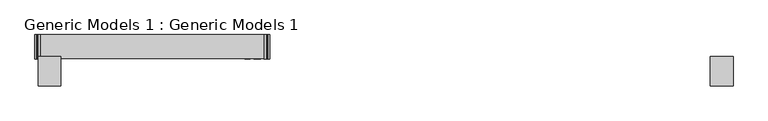
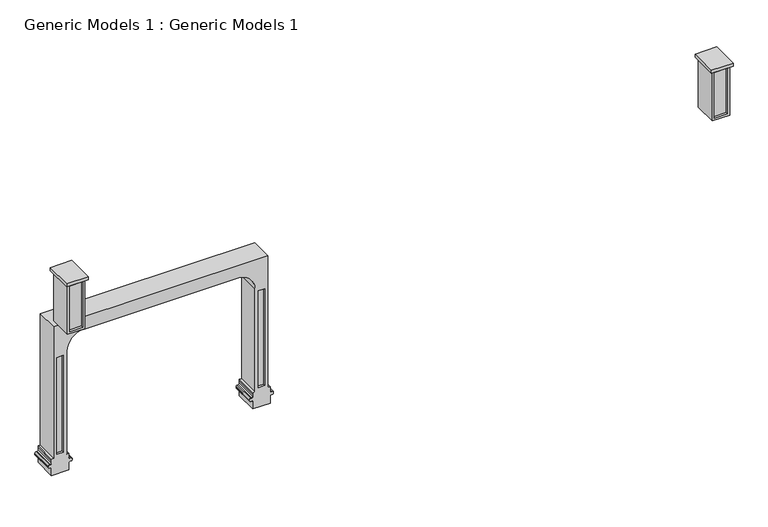
"""IFC4 building model written with IfcOpenShell, lengths in millimetres: proxy geometry, Generic Models 1 : Generic Models 1."""

from ifc_helpers import new_model, si_unit, frame, origin, place, context, project, spatial, polyline, circle_curve, outline, extrude, faceted_brep, source, transform, mapped, element, save
from ifc_brep_helpers import plane_surface, cylinder_surface, revolved_surface, advanced_brep


def generic_models_1_generic_models_1_a6c1d6b2(model_context):
    return source(origin(), model_context, "Body", "SolidModel", [
        advanced_brep(
        [(-3767.7753219, -7793.5697181, 3657.6), (-3767.7753219, -7793.5697181, 406.4), (-3716.9753219, -7793.5697181, 406.4), (-3716.9753219, -7793.5697181, 355.6), (-3716.9753219, -7793.5697181, 304.8), (-3691.5753219, -7793.5697181, 279.4), (-3672.5253219, -7793.5697181, 279.4), (-3640.7753219, -7793.5697181, 247.65), (-3640.7753219, -7793.5697181, 228.6), (-3666.1753219, -7793.5697181, 203.2), (-3695.5632105, -7793.5697181, 203.2), (-3716.9753219, -7793.5697181, 181.7878886), (-3716.9753219, -7793.5697181, 0.0), (-4123.3753219, -7793.5697181, 0.0), (-4123.3753219, -7793.5697181, 181.7878886), (-4144.7874333, -7793.5697181, 203.2), (-4174.1753219, -7793.5697181, 203.2), (-4199.5753219, -7793.5697181, 228.6), (-4199.5753219, -7793.5697181, 247.65), (-4167.8253219, -7793.5697181, 279.4), (-4148.7753219, -7793.5697181, 279.4), (-4123.3753219, -7793.5697181, 304.8), (-4123.3753219, -7793.5697181, 355.6), (-4123.3753219, -7793.5697181, 406.4), (-4072.5753219, -7793.5697181, 406.4), (-4072.5753219, -7793.5697181, 2946.4), (-4478.9753219, -7793.5697181, 3352.8), (-8061.3249265, -7793.5697181, 3352.8), (-8467.7249265, -7793.5697181, 2946.4), (-8467.7249265, -7793.5697181, 406.4), (-8416.9249265, -7793.5697181, 406.4), (-8416.9249265, -7793.5697181, 355.6), (-8416.9249265, -7793.5697181, 304.8), (-8391.5249265, -7793.5697181, 279.4), (-8372.4749265, -7793.5697181, 279.4), (-8340.7249265, -7793.5697181, 247.65), (-8340.7249265, -7793.5697181, 228.6), (-8366.1249265, -7793.5697181, 203.2), (-8395.5128151, -7793.5697181, 203.2), (-8416.9249265, -7793.5697181, 181.7878886), (-8416.9249265, -7793.5697181, 0.0), (-8823.3249265, -7793.5697181, 0.0), (-8823.3249265, -7793.5697181, 181.7878886), (-8844.7370379, -7793.5697181, 203.2), (-8874.1249265, -7793.5697181, 203.2), (-8899.5249265, -7793.5697181, 228.6), (-8899.5249265, -7793.5697181, 247.65), (-8867.7749265, -7793.5697181, 279.4), (-8848.7249265, -7793.5697181, 279.4), (-8823.3249265, -7793.5697181, 304.8), (-8823.3249265, -7793.5697181, 355.6), (-8823.3249265, -7793.5697181, 406.4), (-8772.5249265, -7793.5697181, 406.4), (-8772.5249265, -7793.5697181, 3657.6), (-3767.7753219, -8332.8472664, 3657.6), (-8772.5249265, -8332.8472664, 3657.6), (-8772.5249265, -8332.8472664, 406.4), (-8823.3249265, -8332.8472664, 406.4), (-8823.3249265, -8332.8472664, 355.6), (-8823.3249265, -8332.8472664, 304.8), (-8848.7249265, -8332.8472664, 279.4), (-8867.7749265, -8332.8472664, 279.4), (-8899.5249265, -8332.8472664, 247.65), (-8899.5249265, -8332.8472664, 228.6), (-8874.1249265, -8332.8472664, 203.2), (-8844.7370379, -8332.8472664, 203.2), (-8823.3249265, -8332.8472664, 181.7878886), (-8823.3249265, -8332.8472664, 0.0), (-8416.9249265, -8332.8472664, 0.0), (-8416.9249265, -8332.8472664, 181.7878886), (-8395.5128151, -8332.8472664, 203.2), (-8366.1249265, -8332.8472664, 203.2), (-8340.7249265, -8332.8472664, 228.6), (-8340.7249265, -8332.8472664, 247.65), (-8372.4749265, -8332.8472664, 279.4), (-8391.5249265, -8332.8472664, 279.4), (-8416.9249265, -8332.8472664, 304.8), (-8416.9249265, -8332.8472664, 355.6), (-8416.9249265, -8332.8472664, 406.4), (-8467.7249265, -8332.8472664, 406.4), (-8467.7249265, -8332.8472664, 2946.4), (-8061.3249265, -8332.8472664, 3352.8), (-4478.9753219, -8332.8472664, 3352.8), (-4072.5753219, -8332.8472664, 2946.4), (-4072.5753219, -8332.8472664, 406.4), (-4123.3753219, -8332.8472664, 406.4), (-4123.3753219, -8332.8472664, 355.6), (-4123.3753219, -8332.8472664, 304.8), (-4148.7753219, -8332.8472664, 279.4), (-4167.8253219, -8332.8472664, 279.4), (-4199.5753219, -8332.8472664, 247.65), (-4199.5753219, -8332.8472664, 228.6), (-4174.1753219, -8332.8472664, 203.2), (-4144.7874333, -8332.8472664, 203.2), (-4123.3753219, -8332.8472664, 181.7878886), (-4123.3753219, -8332.8472664, 0.0), (-3716.9753219, -8332.8472664, 0.0), (-3716.9753219, -8332.8472664, 181.7878886), (-3695.5632105, -8332.8472664, 203.2), (-3666.1753219, -8332.8472664, 203.2), (-3640.7753219, -8332.8472664, 228.6), (-3640.7753219, -8332.8472664, 247.65), (-3672.5253219, -8332.8472664, 279.4), (-3691.5753219, -8332.8472664, 279.4), (-3716.9753219, -8332.8472664, 304.8), (-3716.9753219, -8332.8472664, 355.6), (-3716.9753219, -8332.8472664, 406.4), (-3767.7753219, -8332.8472664, 406.4), (-8543.9249265, -8332.8472664, 482.6), (-8696.3249265, -8332.8472664, 482.6), (-8696.3249265, -8332.8472664, 2870.2), (-8543.9249265, -8332.8472664, 2870.2), (-3843.9753219, -8332.8472664, 482.6), (-3996.3753219, -8332.8472664, 482.6), (-3996.3753219, -8332.8472664, 2870.2), (-3843.9753219, -8332.8472664, 2870.2), (-8543.9249265, -8282.0472664, 482.6), (-8543.9249265, -8282.0472664, 2870.2), (-8696.3249265, -8282.0472664, 2870.2), (-8696.3249265, -8282.0472664, 482.6), (-3843.9753219, -8282.0472664, 482.6), (-3843.9753219, -8282.0472664, 2870.2), (-3996.3753219, -8282.0472664, 2870.2), (-3996.3753219, -8282.0472664, 482.6)],
        [
            (0, 1),
            (1, 2),
            (2, 3),
            (3, 4),
            (4, 5, circle_curve(frame((-3691.5753219, -7793.5697181, 304.8), z_axis=(0.0, -1.0, 0.0), x_axis=(1.0, 0.0, 0.0)), 25.4)),
            (5, 6),
            (6, 7, circle_curve(frame((-3672.5253219, -7793.5697181, 247.65), z_axis=(0.0, 1.0, 0.0), x_axis=(1.0, 0.0, 0.0)), 31.75)),
            (7, 8),
            (8, 9, circle_curve(frame((-3666.1753219, -7793.5697181, 228.6), z_axis=(0.0, 1.0, 0.0), x_axis=(1.0, 0.0, 0.0)), 25.4)),
            (9, 10),
            (10, 11, circle_curve(frame((-3695.5632105, -7793.5697181, 181.7878886), z_axis=(0.0, -1.0, 0.0), x_axis=(1.0, 0.0, 0.0)), 21.4121114)),
            (11, 12),
            (12, 13),
            (13, 14),
            (14, 15, circle_curve(frame((-4144.7874333, -7793.5697181, 181.7878886), z_axis=(0.0, -1.0, 0.0), x_axis=(-1.0, 0.0, 0.0)), 21.4121114)),
            (15, 16),
            (16, 17, circle_curve(frame((-4174.1753219, -7793.5697181, 228.6), z_axis=(0.0, 1.0, 0.0), x_axis=(-1.0, 0.0, 0.0)), 25.4)),
            (17, 18),
            (18, 19, circle_curve(frame((-4167.8253219, -7793.5697181, 247.65), z_axis=(0.0, 1.0, 0.0), x_axis=(-1.0, 0.0, 0.0)), 31.75)),
            (19, 20),
            (20, 21, circle_curve(frame((-4148.7753219, -7793.5697181, 304.8), z_axis=(0.0, -1.0, 0.0), x_axis=(-1.0, 0.0, 0.0)), 25.4)),
            (21, 22),
            (22, 23),
            (23, 24),
            (24, 25),
            (25, 26, circle_curve(frame((-4478.9753219, -7793.5697181, 2946.4), z_axis=(0.0, -1.0, 0.0), x_axis=(-1.0, 0.0, 0.0)), 406.4)),
            (26, 27),
            (27, 28, circle_curve(frame((-8061.3249265, -7793.5697181, 2946.4), z_axis=(0.0, -1.0, 0.0), x_axis=(-1.0, 0.0, 0.0)), 406.4)),
            (28, 29),
            (29, 30),
            (30, 31),
            (31, 32),
            (32, 33, circle_curve(frame((-8391.5249265, -7793.5697181, 304.8), z_axis=(0.0, -1.0, 0.0), x_axis=(1.0, 0.0, 0.0)), 25.4)),
            (33, 34),
            (34, 35, circle_curve(frame((-8372.4749265, -7793.5697181, 247.65), z_axis=(0.0, 1.0, 0.0), x_axis=(1.0, 0.0, 0.0)), 31.75)),
            (35, 36),
            (36, 37, circle_curve(frame((-8366.1249265, -7793.5697181, 228.6), z_axis=(0.0, 1.0, 0.0), x_axis=(1.0, 0.0, 0.0)), 25.4)),
            (37, 38),
            (38, 39, circle_curve(frame((-8395.5128151, -7793.5697181, 181.7878886), z_axis=(0.0, -1.0, 0.0), x_axis=(1.0, 0.0, 0.0)), 21.4121114)),
            (39, 40),
            (40, 41),
            (41, 42),
            (42, 43, circle_curve(frame((-8844.7370379, -7793.5697181, 181.7878886), z_axis=(0.0, -1.0, 0.0), x_axis=(-1.0, 0.0, 0.0)), 21.4121114)),
            (43, 44),
            (44, 45, circle_curve(frame((-8874.1249265, -7793.5697181, 228.6), z_axis=(0.0, 1.0, 0.0), x_axis=(-1.0, 0.0, 0.0)), 25.4)),
            (45, 46),
            (46, 47, circle_curve(frame((-8867.7749265, -7793.5697181, 247.65), z_axis=(0.0, 1.0, 0.0), x_axis=(-1.0, 0.0, 0.0)), 31.75)),
            (47, 48),
            (48, 49, circle_curve(frame((-8848.7249265, -7793.5697181, 304.8), z_axis=(0.0, -1.0, 0.0), x_axis=(-1.0, 0.0, 0.0)), 25.4)),
            (49, 50),
            (50, 51),
            (51, 52),
            (52, 53),
            (53, 0),
            (54, 55),
            (55, 56),
            (56, 57),
            (57, 58),
            (58, 59),
            (59, 60, circle_curve(frame((-8848.7249265, -8332.8472664, 304.8), z_axis=(0.0, 1.0, 0.0), x_axis=(-1.0, 0.0, 0.0)), 25.4)),
            (60, 61),
            (61, 62, circle_curve(frame((-8867.7749265, -8332.8472664, 247.65), z_axis=(0.0, -1.0, 0.0), x_axis=(-1.0, 0.0, 0.0)), 31.75)),
            (62, 63),
            (63, 64, circle_curve(frame((-8874.1249265, -8332.8472664, 228.6), z_axis=(0.0, -1.0, 0.0), x_axis=(-1.0, 0.0, 0.0)), 25.4)),
            (64, 65),
            (65, 66, circle_curve(frame((-8844.7370379, -8332.8472664, 181.7878886), z_axis=(0.0, 1.0, 0.0), x_axis=(-1.0, 0.0, 0.0)), 21.4121114)),
            (66, 67),
            (67, 68),
            (68, 69),
            (69, 70, circle_curve(frame((-8395.5128151, -8332.8472664, 181.7878886), z_axis=(0.0, 1.0, 0.0), x_axis=(1.0, 0.0, 0.0)), 21.4121114)),
            (70, 71),
            (71, 72, circle_curve(frame((-8366.1249265, -8332.8472664, 228.6), z_axis=(0.0, -1.0, 0.0), x_axis=(1.0, 0.0, 0.0)), 25.4)),
            (72, 73),
            (73, 74, circle_curve(frame((-8372.4749265, -8332.8472664, 247.65), z_axis=(0.0, -1.0, 0.0), x_axis=(1.0, 0.0, 0.0)), 31.75)),
            (74, 75),
            (75, 76, circle_curve(frame((-8391.5249265, -8332.8472664, 304.8), z_axis=(0.0, 1.0, 0.0), x_axis=(1.0, 0.0, 0.0)), 25.4)),
            (76, 77),
            (77, 78),
            (78, 79),
            (79, 80),
            (80, 81, circle_curve(frame((-8061.3249265, -8332.8472664, 2946.4), z_axis=(0.0, 1.0, 0.0), x_axis=(-1.0, 0.0, 0.0)), 406.4)),
            (81, 82),
            (82, 83, circle_curve(frame((-4478.9753219, -8332.8472664, 2946.4), z_axis=(0.0, 1.0, 0.0), x_axis=(-1.0, 0.0, 0.0)), 406.4)),
            (83, 84),
            (84, 85),
            (85, 86),
            (86, 87),
            (87, 88, circle_curve(frame((-4148.7753219, -8332.8472664, 304.8), z_axis=(0.0, 1.0, 0.0), x_axis=(-1.0, 0.0, 0.0)), 25.4)),
            (88, 89),
            (89, 90, circle_curve(frame((-4167.8253219, -8332.8472664, 247.65), z_axis=(0.0, -1.0, 0.0), x_axis=(-1.0, 0.0, 0.0)), 31.75)),
            (90, 91),
            (91, 92, circle_curve(frame((-4174.1753219, -8332.8472664, 228.6), z_axis=(0.0, -1.0, 0.0), x_axis=(-1.0, 0.0, 0.0)), 25.4)),
            (92, 93),
            (93, 94, circle_curve(frame((-4144.7874333, -8332.8472664, 181.7878886), z_axis=(0.0, 1.0, 0.0), x_axis=(-1.0, 0.0, 0.0)), 21.4121114)),
            (94, 95),
            (95, 96),
            (96, 97),
            (97, 98, circle_curve(frame((-3695.5632105, -8332.8472664, 181.7878886), z_axis=(0.0, 1.0, 0.0), x_axis=(1.0, 0.0, 0.0)), 21.4121114)),
            (98, 99),
            (99, 100, circle_curve(frame((-3666.1753219, -8332.8472664, 228.6), z_axis=(0.0, -1.0, 0.0), x_axis=(1.0, 0.0, 0.0)), 25.4)),
            (100, 101),
            (101, 102, circle_curve(frame((-3672.5253219, -8332.8472664, 247.65), z_axis=(0.0, -1.0, 0.0), x_axis=(1.0, 0.0, 0.0)), 31.75)),
            (102, 103),
            (103, 104, circle_curve(frame((-3691.5753219, -8332.8472664, 304.8), z_axis=(0.0, 1.0, 0.0), x_axis=(1.0, 0.0, 0.0)), 25.4)),
            (104, 105),
            (105, 106),
            (106, 107),
            (107, 54),
            (108, 109),
            (109, 110),
            (110, 111),
            (111, 108),
            (112, 113),
            (113, 114),
            (114, 115),
            (115, 112),
            (0, 54),
            (107, 1),
            (106, 2),
            (105, 3),
            (104, 4),
            (103, 5),
            (102, 6),
            (101, 7),
            (100, 8),
            (99, 9),
            (98, 10),
            (97, 11),
            (96, 12),
            (95, 13),
            (94, 14),
            (93, 15),
            (92, 16),
            (91, 17),
            (90, 18),
            (89, 19),
            (88, 20),
            (87, 21),
            (86, 22),
            (85, 23),
            (84, 24),
            (83, 25),
            (82, 26),
            (81, 27),
            (80, 28),
            (79, 29),
            (52, 56),
            (55, 53),
            (78, 30),
            (77, 31),
            (76, 32),
            (75, 33),
            (74, 34),
            (73, 35),
            (72, 36),
            (71, 37),
            (70, 38),
            (69, 39),
            (68, 40),
            (67, 41),
            (66, 42),
            (65, 43),
            (64, 44),
            (63, 45),
            (62, 46),
            (61, 47),
            (60, 48),
            (59, 49),
            (58, 50),
            (57, 51),
            (116, 117),
            (117, 118),
            (118, 119),
            (119, 116),
            (120, 121),
            (121, 122),
            (122, 123),
            (123, 120),
            (119, 109),
            (108, 116),
            (118, 110),
            (117, 111),
            (123, 113),
            (112, 120),
            (122, 114),
            (121, 115),
        ],
        [
            plane_surface(frame((-3767.7753219, -7793.5697181, 3657.6), z_axis=(0.0, 1.0, 0.0), x_axis=(0.0, 0.0, -1.0))),
            plane_surface(frame((-3767.7753219, -8332.8472664, 3657.6), z_axis=(0.0, -1.0, 0.0), x_axis=(0.0, 0.0, 1.0))),
            plane_surface(frame((-3767.7753219, -7793.5697181, 3657.6), z_axis=(1.0, 0.0, 0.0), x_axis=(0.0, -1.0, 0.0))),
            plane_surface(frame((-3767.7753219, -7793.5697181, 406.4), z_axis=(0.0, 0.0, 1.0), x_axis=(0.0, -1.0, 0.0))),
            plane_surface(frame((-3716.9753219, -7793.5697181, 406.4), z_axis=(1.0, 0.0, 0.0), x_axis=(0.0, -1.0, 0.0))),
            plane_surface(frame((-3716.9753219, -7793.5697181, 355.6), z_axis=(1.0, 0.0, 0.0), x_axis=(0.0, -1.0, 0.0))),
            revolved_surface(polyline([(-3666.1753218999997, -8332.8472664, 304.8), (-3666.1753218999997, -7793.5697181, 304.8)]), (-3691.5753219, -8332.8472664, 304.8), (0.0, -1.0, 0.0)),
            plane_surface(frame((-3691.5753219, -7793.5697181, 279.4), z_axis=(0.0, 0.0, 1.0), x_axis=(0.0, -1.0, 0.0))),
            cylinder_surface(frame((-3672.5253219, -8332.8472664, 247.65), z_axis=(0.0, 1.0, 0.0), x_axis=(1.0, 0.0, 0.0)), 31.75),
            plane_surface(frame((-3640.7753219, -7793.5697181, 247.65), z_axis=(1.0, 0.0, 0.0), x_axis=(0.0, -1.0, 0.0))),
            cylinder_surface(frame((-3666.1753219, -8332.8472664, 228.6), z_axis=(0.0, 1.0, 0.0), x_axis=(1.0, 0.0, 0.0)), 25.4),
            plane_surface(frame((-3666.1753219, -7793.5697181, 203.2), z_axis=(0.0, 0.0, -1.0), x_axis=(0.0, -1.0, 0.0))),
            revolved_surface(polyline([(-3674.1510991, -8332.8472664, 181.7878886), (-3674.1510991, -7793.5697181, 181.7878886)]), (-3695.5632105, -8332.8472664, 181.7878886), (0.0, -1.0, 0.0)),
            plane_surface(frame((-3716.9753219, -7793.5697181, 181.7878886), z_axis=(1.0, 0.0, 0.0), x_axis=(0.0, -1.0, 0.0))),
            plane_surface(frame((-3716.9753219, -7793.5697181, 0.0), z_axis=(0.0, 0.0, -1.0), x_axis=(0.0, -1.0, 0.0))),
            plane_surface(frame((-4123.3753219, -7793.5697181, 0.0), z_axis=(-1.0, 0.0, 0.0), x_axis=(0.0, -1.0, 0.0))),
            revolved_surface(polyline([(-4166.1995447, -8332.8472664, 181.7878886), (-4166.1995447, -7793.5697181, 181.7878886)]), (-4144.7874333, -8332.8472664, 181.7878886), (0.0, -1.0, 0.0)),
            plane_surface(frame((-4144.7874333, -7793.5697181, 203.2), z_axis=(0.0, 0.0, -1.0), x_axis=(0.0, -1.0, 0.0))),
            cylinder_surface(frame((-4174.1753219, -8332.8472664, 228.6), z_axis=(0.0, 1.0, 0.0), x_axis=(-1.0, 0.0, 0.0)), 25.4),
            plane_surface(frame((-4199.5753219, -7793.5697181, 228.6), z_axis=(-1.0, 0.0, 0.0), x_axis=(0.0, -1.0, 0.0))),
            cylinder_surface(frame((-4167.8253219, -8332.8472664, 247.65), z_axis=(0.0, 1.0, 0.0), x_axis=(-1.0, 0.0, 0.0)), 31.75),
            plane_surface(frame((-4167.8253219, -7793.5697181, 279.4), z_axis=(0.0, 0.0, 1.0), x_axis=(0.0, -1.0, 0.0))),
            revolved_surface(polyline([(-4174.175321899999, -8332.8472664, 304.8), (-4174.175321899999, -7793.5697181, 304.8)]), (-4148.7753219, -8332.8472664, 304.8), (0.0, -1.0, 0.0)),
            plane_surface(frame((-4123.3753219, -7793.5697181, 304.8), z_axis=(-1.0, 0.0, 0.0), x_axis=(0.0, -1.0, 0.0))),
            plane_surface(frame((-4123.3753219, -7793.5697181, 355.6), z_axis=(-1.0, 0.0, 0.0), x_axis=(0.0, -1.0, 0.0))),
            plane_surface(frame((-4123.3753219, -7793.5697181, 406.4), z_axis=(0.0, 0.0, 1.0), x_axis=(0.0, -1.0, 0.0))),
            plane_surface(frame((-4072.5753219, -7793.5697181, 406.4), z_axis=(-1.0, 0.0, 0.0), x_axis=(0.0, -1.0, 0.0))),
            revolved_surface(polyline([(-4885.3753219, -8332.8472664, 2946.4), (-4885.3753219, -7793.5697181, 2946.4)]), (-4478.9753219, -8332.8472664, 2946.4), (0.0, -1.0, 0.0)),
            plane_surface(frame((-4478.9753219, -7793.5697181, 3352.8), z_axis=(0.0, 0.0, -1.0), x_axis=(0.0, -1.0, 0.0))),
            revolved_surface(polyline([(-8467.724926500001, -8332.8472664, 2946.4), (-8467.724926500001, -7793.5697181, 2946.4)]), (-8061.3249265, -8332.8472664, 2946.4), (0.0, -1.0, 0.0)),
            plane_surface(frame((-8467.7249265, -7793.5697181, 2946.4), z_axis=(1.0, 0.0, 0.0), x_axis=(0.0, -1.0, 0.0))),
            plane_surface(frame((-8772.5249265, -7793.5697181, 406.4), z_axis=(-1.0, 0.0, 0.0), x_axis=(0.0, -1.0, 0.0))),
            plane_surface(frame((-8772.5249265, -7793.5697181, 3657.6), z_axis=(0.0, 0.0, 1.0), x_axis=(0.0, -1.0, 0.0))),
            plane_surface(frame((-8467.7249265, -7793.5697181, 406.4), z_axis=(0.0, 0.0, 1.0), x_axis=(0.0, -1.0, 0.0))),
            plane_surface(frame((-8416.9249265, -7793.5697181, 406.4), z_axis=(1.0, 0.0, 0.0), x_axis=(0.0, -1.0, 0.0))),
            plane_surface(frame((-8416.9249265, -7793.5697181, 355.6), z_axis=(1.0, 0.0, 0.0), x_axis=(0.0, -1.0, 0.0))),
            revolved_surface(polyline([(-8366.1249265, -8332.8472664, 304.8), (-8366.1249265, -7793.5697181, 304.8)]), (-8391.5249265, -8332.8472664, 304.8), (0.0, -1.0, 0.0)),
            plane_surface(frame((-8391.5249265, -7793.5697181, 279.4), z_axis=(0.0, 0.0, 1.0), x_axis=(0.0, -1.0, 0.0))),
            cylinder_surface(frame((-8372.4749265, -8332.8472664, 247.65), z_axis=(0.0, 1.0, 0.0), x_axis=(1.0, 0.0, 0.0)), 31.75),
            plane_surface(frame((-8340.7249265, -7793.5697181, 247.65), z_axis=(1.0, 0.0, 0.0), x_axis=(0.0, -1.0, 0.0))),
            cylinder_surface(frame((-8366.1249265, -8332.8472664, 228.6), z_axis=(0.0, 1.0, 0.0), x_axis=(1.0, 0.0, 0.0)), 25.4),
            plane_surface(frame((-8366.1249265, -7793.5697181, 203.2), z_axis=(0.0, 0.0, -1.0), x_axis=(0.0, -1.0, 0.0))),
            revolved_surface(polyline([(-8374.1007037, -8332.8472664, 181.7878886), (-8374.1007037, -7793.5697181, 181.7878886)]), (-8395.5128151, -8332.8472664, 181.7878886), (0.0, -1.0, 0.0)),
            plane_surface(frame((-8416.9249265, -7793.5697181, 181.7878886), z_axis=(1.0, 0.0, 0.0), x_axis=(0.0, -1.0, 0.0))),
            plane_surface(frame((-8416.9249265, -7793.5697181, 0.0), z_axis=(0.0, 0.0, -1.0), x_axis=(0.0, -1.0, 0.0))),
            plane_surface(frame((-8823.3249265, -7793.5697181, 0.0), z_axis=(-1.0, 0.0, 0.0), x_axis=(0.0, -1.0, 0.0))),
            revolved_surface(polyline([(-8866.149149300001, -8332.8472664, 181.7878886), (-8866.149149300001, -7793.5697181, 181.7878886)]), (-8844.7370379, -8332.8472664, 181.7878886), (0.0, -1.0, 0.0)),
            plane_surface(frame((-8844.7370379, -7793.5697181, 203.2), z_axis=(0.0, 0.0, -1.0), x_axis=(0.0, -1.0, 0.0))),
            cylinder_surface(frame((-8874.1249265, -8332.8472664, 228.6), z_axis=(0.0, 1.0, 0.0), x_axis=(-1.0, 0.0, 0.0)), 25.4),
            plane_surface(frame((-8899.5249265, -7793.5697181, 228.6), z_axis=(-1.0, 0.0, 0.0), x_axis=(0.0, -1.0, 0.0))),
            cylinder_surface(frame((-8867.7749265, -8332.8472664, 247.65), z_axis=(0.0, 1.0, 0.0), x_axis=(-1.0, 0.0, 0.0)), 31.75),
            plane_surface(frame((-8867.7749265, -7793.5697181, 279.4), z_axis=(0.0, 0.0, 1.0), x_axis=(0.0, -1.0, 0.0))),
            revolved_surface(polyline([(-8874.124926499999, -8332.8472664, 304.8), (-8874.124926499999, -7793.5697181, 304.8)]), (-8848.7249265, -8332.8472664, 304.8), (0.0, -1.0, 0.0)),
            plane_surface(frame((-8823.3249265, -7793.5697181, 304.8), z_axis=(-1.0, 0.0, 0.0), x_axis=(0.0, -1.0, 0.0))),
            plane_surface(frame((-8823.3249265, -7793.5697181, 355.6), z_axis=(-1.0, 0.0, 0.0), x_axis=(0.0, -1.0, 0.0))),
            plane_surface(frame((-8823.3249265, -7793.5697181, 406.4), z_axis=(0.0, 0.0, 1.0), x_axis=(0.0, -1.0, 0.0))),
            plane_surface(frame((-8696.3249265, -8282.0472664, 482.6), z_axis=(0.0, -1.0, 0.0), x_axis=(-1.0, 0.0, 0.0))),
            plane_surface(frame((-8543.9249265, -8282.0472664, 482.6), z_axis=(0.0, 0.0, 1.0), x_axis=(0.0, -1.0, 0.0))),
            plane_surface(frame((-8696.3249265, -8282.0472664, 482.6), z_axis=(1.0, 0.0, 0.0), x_axis=(0.0, -1.0, 0.0))),
            plane_surface(frame((-8696.3249265, -8282.0472664, 2870.2), z_axis=(0.0, 0.0, -1.0), x_axis=(0.0, -1.0, 0.0))),
            plane_surface(frame((-8543.9249265, -8282.0472664, 2870.2), z_axis=(-1.0, 0.0, 0.0), x_axis=(0.0, -1.0, 0.0))),
            plane_surface(frame((-3843.9753219, -8282.0472664, 482.6), z_axis=(0.0, 0.0, 1.0), x_axis=(0.0, -1.0, 0.0))),
            plane_surface(frame((-3996.3753219, -8282.0472664, 482.6), z_axis=(1.0, 0.0, 0.0), x_axis=(0.0, -1.0, 0.0))),
            plane_surface(frame((-3996.3753219, -8282.0472664, 2870.2), z_axis=(0.0, 0.0, -1.0), x_axis=(0.0, -1.0, 0.0))),
            plane_surface(frame((-3843.9753219, -8282.0472664, 2870.2), z_axis=(-1.0, 0.0, 0.0), x_axis=(0.0, -1.0, 0.0))),
        ],
        [
            (0, [[1, 2, 3, 4, 5, 6, 7, 8, 9, 10, 11, 12, 13, 14, 15, 16, 17, 18, 19, 20, 21, 22, 23, 24, 25, 26, 27, 28, 29, 30, 31, 32, 33, 34, 35, 36, 37, 38, 39, 40, 41, 42, 43, 44, 45, 46, 47, 48, 49, 50, 51, 52, 53, 54]]),
            (1, [[55, 56, 57, 58, 59, 60, 61, 62, 63, 64, 65, 66, 67, 68, 69, 70, 71, 72, 73, 74, 75, 76, 77, 78, 79, 80, 81, 82, 83, 84, 85, 86, 87, 88, 89, 90, 91, 92, 93, 94, 95, 96, 97, 98, 99, 100, 101, 102, 103, 104, 105, 106, 107, 108], [109, 110, 111, 112], [113, 114, 115, 116]]),
            (2, [[-1, 117, -108, 118]]),
            (3, [[-2, -118, -107, 119]]),
            (4, [[-3, -119, -106, 120]]),
            (5, [[-4, -120, -105, 121]]),
            (6, [[-5, -121, -104, 122]]),
            (7, [[-6, -122, -103, 123]]),
            (8, [[-7, -123, -102, 124]]),
            (9, [[-8, -124, -101, 125]]),
            (10, [[-9, -125, -100, 126]]),
            (11, [[-10, -126, -99, 127]]),
            (12, [[-11, -127, -98, 128]]),
            (13, [[-12, -128, -97, 129]]),
            (14, [[-13, -129, -96, 130]]),
            (15, [[-14, -130, -95, 131]]),
            (16, [[-15, -131, -94, 132]]),
            (17, [[-16, -132, -93, 133]]),
            (18, [[-17, -133, -92, 134]]),
            (19, [[-18, -134, -91, 135]]),
            (20, [[-19, -135, -90, 136]]),
            (21, [[-20, -136, -89, 137]]),
            (22, [[-21, -137, -88, 138]]),
            (23, [[-22, -138, -87, 139]]),
            (24, [[-23, -139, -86, 140]]),
            (25, [[-24, -140, -85, 141]]),
            (26, [[-25, -141, -84, 142]]),
            (27, [[-26, -142, -83, 143]]),
            (28, [[-27, -143, -82, 144]]),
            (29, [[-28, -144, -81, 145]]),
            (30, [[-29, -145, -80, 146]]),
            (31, [[-53, 147, -56, 148]]),
            (32, [[-54, -148, -55, -117]]),
            (33, [[-30, -146, -79, 149]]),
            (34, [[-31, -149, -78, 150]]),
            (35, [[-32, -150, -77, 151]]),
            (36, [[-33, -151, -76, 152]]),
            (37, [[-34, -152, -75, 153]]),
            (38, [[-35, -153, -74, 154]]),
            (39, [[-36, -154, -73, 155]]),
            (40, [[-37, -155, -72, 156]]),
            (41, [[-38, -156, -71, 157]]),
            (42, [[-39, -157, -70, 158]]),
            (43, [[-40, -158, -69, 159]]),
            (44, [[-41, -159, -68, 160]]),
            (45, [[-42, -160, -67, 161]]),
            (46, [[-43, -161, -66, 162]]),
            (47, [[-44, -162, -65, 163]]),
            (48, [[-45, -163, -64, 164]]),
            (49, [[-46, -164, -63, 165]]),
            (50, [[-47, -165, -62, 166]]),
            (51, [[-48, -166, -61, 167]]),
            (52, [[-49, -167, -60, 168]]),
            (53, [[-50, -168, -59, 169]]),
            (54, [[-51, -169, -58, 170]]),
            (55, [[-52, -170, -57, -147]]),
            (56, [[171, 172, 173, 174]]),
            (56, [[175, 176, 177, 178]]),
            (57, [[-174, 179, -109, 180]]),
            (58, [[-173, 181, -110, -179]]),
            (59, [[-172, 182, -111, -181]]),
            (60, [[-171, -180, -112, -182]]),
            (61, [[-178, 183, -113, 184]]),
            (62, [[-177, 185, -114, -183]]),
            (63, [[-176, 186, -115, -185]]),
            (64, [[-175, -184, -116, -186]]),
        ],
    ),
        faceted_brep([(-8772.5249265, -8891.6472664, 5029.2), (-8366.1249265, -8891.6472664, 5029.2), (-8366.1249265, -8332.8472664, 5029.2), (-8772.5249265, -8332.8472664, 5029.2), (-8772.5249265, -8891.6472664, 3810.0), (-8772.5249265, -8332.8472664, 3810.0), (-8366.1249265, -8332.8472664, 3810.0), (-8366.1249265, -8891.6472664, 3810.0), (-8416.9249265, -8891.6472664, 4978.4), (-8416.9249265, -8891.6472664, 3860.8), (-8721.7249265, -8891.6472664, 3860.8), (-8721.7249265, -8891.6472664, 4978.4), (-8416.9249265, -8840.8472664, 4978.4), (-8721.7249265, -8840.8472664, 4978.4), (-8721.7249265, -8840.8472664, 3860.8), (-8416.9249265, -8840.8472664, 3860.8)], [[[0, 1, 2, 3]], [[4, 5, 6, 7]], [[1, 0, 4, 7], [8, 9, 10, 11]], [[2, 1, 7, 6]], [[3, 2, 6, 5]], [[0, 3, 5, 4]], [[12, 13, 14, 15]], [[12, 15, 9, 8]], [[15, 14, 10, 9]], [[14, 13, 11, 10]], [[13, 12, 8, 11]]]),
        faceted_brep([(6289.6750735, -8891.6472664, 5029.2), (6696.0750735, -8891.6472664, 5029.2), (6696.0750735, -8332.8472664, 5029.2), (6289.6750735, -8332.8472664, 5029.2), (6289.6750735, -8891.6472664, 3810.0), (6289.6750735, -8332.8472664, 3810.0), (6696.0750735, -8332.8472664, 3810.0), (6696.0750735, -8891.6472664, 3810.0), (6645.2750735, -8891.6472664, 4978.4), (6645.2750735, -8891.6472664, 3860.8), (6340.4750735, -8891.6472664, 3860.8), (6340.4750735, -8891.6472664, 4978.4), (6645.2750735, -8840.8472664, 4978.4), (6340.4750735, -8840.8472664, 4978.4), (6340.4750735, -8840.8472664, 3860.8), (6645.2750735, -8840.8472664, 3860.8)], [[[0, 1, 2, 3]], [[4, 5, 6, 7]], [[1, 0, 4, 7], [8, 9, 10, 11]], [[2, 1, 7, 6]], [[3, 2, 6, 5]], [[0, 3, 5, 4]], [[12, 13, 14, 15]], [[12, 15, 9, 8]], [[15, 14, 10, 9]], [[14, 13, 11, 10]], [[13, 12, 8, 11]]]),
        extrude(outline(polyline([(-8315.3249265, -8282.0472664), (-8315.3249265, -8942.4472664), (-8823.3249265, -8942.4472664), (-8823.3249265, -8282.0472664), (-8315.3249265, -8282.0472664)])), frame((0.0, 0.0, 5029.2), z_axis=(0.0, 0.0, 1.0), x_axis=(1.0, 0.0, 0.0)), (0.0, 0.0, 1.0), 76.2),
        extrude(outline(polyline([(6746.8750735, -8282.0472664), (6746.8750735, -8942.4472664), (6238.8750735, -8942.4472664), (6238.8750735, -8282.0472664), (6746.8750735, -8282.0472664)])), frame((0.0, 0.0, 5029.2), z_axis=(0.0, 0.0, 1.0), x_axis=(1.0, 0.0, 0.0)), (0.0, 0.0, 1.0), 76.2),
    ])


if __name__ == "__main__":
    model = new_model("IFC4")
    model_context = context("Model", 3, world=origin())
    ifc_project = project(units=[si_unit("LENGTHUNIT", "METRE", prefix="MILLI")], contexts=[model_context])
    site = spatial("IfcSite", under=ifc_project)
    building = spatial("IfcBuilding", under=site)
    placement = place(None, origin())
    generic_models_1_generic_models_1_shape = generic_models_1_generic_models_1_a6c1d6b2(model_context)
    element("IfcBuildingElementProxy", 1, Name="Generic Models 1 : Generic Models 1", ObjectType="Generic Models 1 : Generic Models 1", at=placement, inside=building, context=model_context, shape_type="MappedRepresentation", body=[
        mapped(generic_models_1_generic_models_1_shape, transform((0.0, 0.0, 0.0), x_axis=(1.0, 0.0, 0.0), y_axis=(0.0, 1.0, 0.0), z_axis=(0.0, 0.0, 1.0))),
    ])
    save(model, "model.ifc")

# Revit data of these elements
# Element 1 (IfcBuildingElementProxy, "Generic Models 1 : Generic Models 1")
#   Materials on its faces: "Laminate, Ivory, Matte", "Earth"
# Materials
#   "Laminate, Ivory, Matte": class "Plastic", colour RGB 247 247 239, transparency 0, Description = "Plastic Laminate - Ivory, Matte", Cost = 0
#   "Earth": class "Generic", colour RGB 97 75 62, transparency 0, Description = "Soil", Cost = 0
